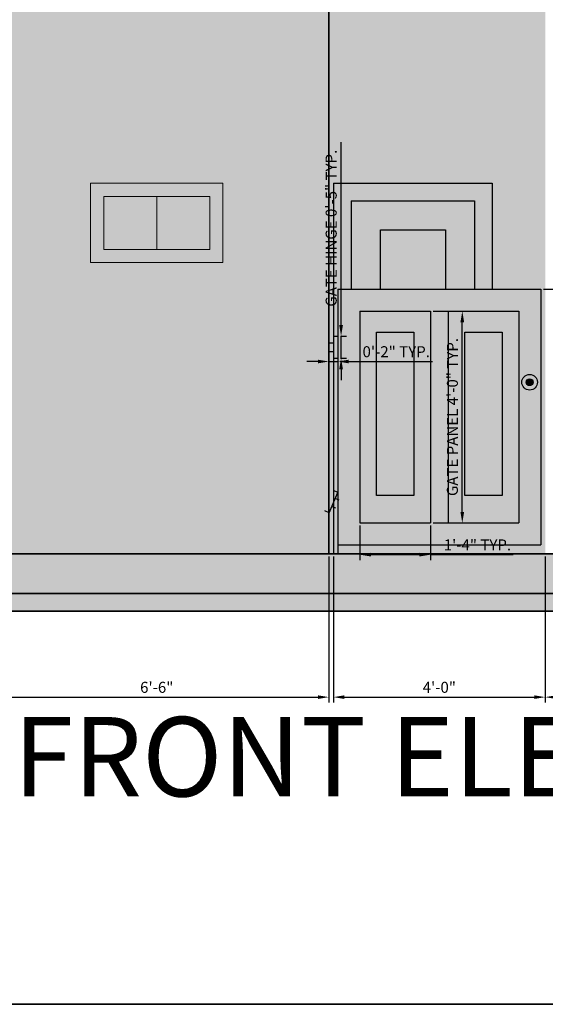
# Model space of a CAD drawing. Units: inches. Extents: x 2150 to 10686, y 1035 to 5077.
# Tile 6 of 12: x 6249 to 6368, y 4201 to 4425. Entities that reach past the tile are written whole.
import ezdxf

# ---------------------------------------------------------------- set-up
doc = ezdxf.new("R2010")
doc.units = ezdxf.units.IN
for name, color, linetype, lineweight in [('A-ANNO-DIMS', 2, 'Continuous', 18), ('A-ANNO-TITL', 3, 'Continuous', 35), ('A-ANNO-TTLB', 7, 'Continuous', 35), ('A-ELEV', 7, 'Continuous', 35), ('A-ELEV-BASE-PATT', 251, 'Continuous', 13), ('A-ELEV-DOOR', 7, 'Continuous', 25), ('A-ELEV-DOOR-PATT', 17, 'Continuous', 13), ('A-ELEV-GLAZ', 7, 'Continuous', 18), ('A-ELEV-METL-PATT', 252, 'Continuous', 13)]:
    doc.layers.add(name, color=color, linetype=linetype, lineweight=lineweight)
doc.layers.add('A-ELEV-GLAZ-PATT', color=141, linetype='Continuous', lineweight=13, true_color=0xadddf7)
doc.layers.add('A-ELEV-PATT', color=253, linetype='Continuous', lineweight=13, true_color=0xa5adc8)
doc.styles.get("Standard").update_dxf_attribs({"font": 'arial.ttf'})
doc.dimstyles.new('ISO-25', dxfattribs={"dimtxt": 2.5, "dimasz": 2.5, "dimexe": 1.25, "dimexo": 0.625, "dimtad": 1, "dimdec": 0, "dimlunit": 3, "dimtxsty": 'Standard', "dimcen": 2.5, "dimadec": 0, "dimazin": 0, "dimtfac": 1, "dimtdec": 0, "dimtmove": 0, "dimatfit": 3, "dimfxl": 1, "dimarcsym": 0})

# ---------------------------------------------------------------- blocks, each defined once
blk = doc.blocks.new('GATE-INSET-PANEL-16')
for p, q in [((-0.0003365621996636, 48.00046013132396), (15.99966343780033, 48.00046013132396)), ((-0.0003365621987541, 48.00046013132396), (-0.0003365622005731, 0.0004601313230523)), ((15.99966343780033, 48.00046013132396), (15.99966343780033, 0.0004601313239618)), ((-0.0003365622005731, 0.0004601313239618), (15.99966343780033, 0.0004601313239618))]:
    blk.add_line(p, q)
blk.add_lwpolyline([(3.788000571435077, 43.25048342382524), (12.21132630416559, 43.25048342382524), (12.21132630416559, 6.206833629573338), (3.788000571435077, 6.206833629573338)], close=True)
blk = doc.blocks.new('GATE-HINGE-5IN')
for p, q in [((0.9996634378003363, 5.000328444739352), (1.999663437801245, 5.000328444739352)), ((0.9996634378003363, 5.000328444739352), (0.9996634378003363, 0.0003284447393526)), ((-0.0003365622005731, 3.500328444739352), (0.9996634378003363, 3.500328444739352)), ((-0.0003365622005731, 1.500328444739352), (0.9996634378003363, 1.500328444739352)), ((0.9996634378003363, 0.0003284447402621), (1.999663437801245, 0.0003284447393526))]:
    blk.add_line(p, q)
blk = doc.blocks.new('*D72')
at = {"layer": 'A-ANNO-DIMS', "color": 0, "lineweight": -2, "transparency": 16777216}
for p, q in [((6342.232663437805, 4358.484460131326), (6350.057663437808, 4358.484460131326)), ((6348.807663437807, 4312.984460131325), (6348.807663437807, 4355.984460131327)), ((6342.232663437805, 4310.484460131325), (6350.057663437808, 4310.484460131325))]:
    blk.add_line(p, q, dxfattribs=at)
at = {"layer": 'A-ANNO-DIMS', "color": 0, "transparency": 16777216}
for points in [[(6348.39099677114, 4355.984460131327), (6349.224330104474, 4355.984460131327), (6348.807663437807, 4358.484460131326)], [(6348.39099677114, 4312.984460131325), (6349.224330104474, 4312.984460131325), (6348.807663437807, 4310.484460131325)]]:
    blk.add_solid(points, dxfattribs=at)
at = {"layer": 'Defpoints', "color": 0, "transparency": 16777216}
for p in [(6341.607663437804, 4358.484460131326), (6348.807663437807, 4358.484460131326), (6341.607663437804, 4310.484460131325)]:
    blk.add_point(p, dxfattribs=at)
at = {"layer": 'A-ANNO-DIMS', "color": 0, "transparency": 16777216, "insert": (6346.8900304228, 4334.484460131323), "char_height": 2.5, "attachment_point": 5, "rotation": 90}
blk.add_mtext('GATE PANEL 4\'-0" TYP.', dxfattribs=at)
blk = doc.blocks.new('*D73')
at = {"layer": 'A-ANNO-DIMS', "color": 0, "lineweight": -2, "transparency": 16777216}
for p, q in [((6325.6076634378, 4309.859460131323), (6325.6076634378, 4302.034460131323)), ((6341.607663437801, 4309.859460131323), (6341.607663437801, 4302.034460131323)), ((6328.107663437799, 4303.284460131323), (6339.1076634378, 4303.284460131323)), ((6341.607663437801, 4303.284460131323), (6360.361074079001, 4303.284460131323))]:
    blk.add_line(p, q, dxfattribs=at)
at = {"layer": 'A-ANNO-DIMS', "color": 0, "transparency": 16777216}
for points in [[(6328.107663437799, 4303.70112679799), (6328.107663437799, 4302.867793464656), (6325.6076634378, 4303.284460131323)], [(6339.1076634378, 4303.70112679799), (6339.1076634378, 4302.867793464656), (6341.607663437801, 4303.284460131323)]]:
    blk.add_solid(points, dxfattribs=at)
at = {"layer": 'Defpoints', "color": 0, "transparency": 16777216}
for p in [(6325.6076634378, 4310.484460131323), (6341.607663437801, 4310.484460131323), (6341.607663437801, 4303.284460131323)]:
    blk.add_point(p, dxfattribs=at)
at = {"layer": 'A-ANNO-DIMS', "color": 0, "transparency": 16777216, "insert": (6352.2343687584, 4305.165428753425), "char_height": 2.5, "attachment_point": 5}
blk.add_mtext('1\'-4" TYP.', dxfattribs=at)
blk = doc.blocks.new('*D76')
at = {"layer": 'A-ANNO-DIMS', "color": 0, "lineweight": -2, "transparency": 16777216}
for p, q in [((6321.35766343781, 4355.313328444741), (6321.35766343781, 4396.771377557974)), ((6321.232663437806, 4352.813328444741), (6322.60766343781, 4352.813328444741)), ((6321.35766343781, 4347.813328444741), (6321.35766343781, 4352.813328444741)), ((6321.232663437806, 4347.813328444741), (6322.60766343781, 4347.813328444741)), ((6321.35766343781, 4345.313328444741), (6321.35766343781, 4342.813328444741))]:
    blk.add_line(p, q, dxfattribs=at)
at = {"layer": 'A-ANNO-DIMS', "color": 0, "transparency": 16777216}
for points in [[(6320.940996771143, 4355.313328444741), (6321.774330104477, 4355.313328444741), (6321.35766343781, 4352.813328444741)], [(6320.940996771143, 4345.313328444741), (6321.774330104477, 4345.313328444741), (6321.35766343781, 4347.813328444741)]]:
    blk.add_solid(points, dxfattribs=at)
at = {"layer": 'Defpoints', "color": 0, "transparency": 16777216}
for p in [(6320.607663437806, 4352.813328444741), (6321.35766343781, 4352.813328444741), (6320.607663437806, 4347.813328444741)]:
    blk.add_point(p, dxfattribs=at)
at = {"layer": 'A-ANNO-DIMS', "color": 0, "transparency": 16777216, "insert": (6319.440030422802, 4377.292353001354), "char_height": 2.5, "attachment_point": 5, "rotation": 90}
blk.add_mtext('GATE HINGE 0\'-5" TYP.', dxfattribs=at)
blk = doc.blocks.new('*D77')
at = {"layer": 'A-ANNO-DIMS', "color": 0, "lineweight": -2, "transparency": 16777216}
for p, q in [((6316.107663437801, 4347.063328444739), (6313.6076634378, 4347.063328444739)), ((6318.6076634378, 4347.188328444739), (6318.6076634378, 4345.813328444739)), ((6318.6076634378, 4347.063328444739), (6320.607663437802, 4347.063328444739)), ((6320.607663437802, 4347.188328444739), (6320.607663437802, 4345.813328444739)), ((6323.107663437802, 4347.063328444739), (6342.09640832184, 4347.063328444739))]:
    blk.add_line(p, q, dxfattribs=at)
at = {"layer": 'A-ANNO-DIMS', "color": 0, "transparency": 16777216}
for points in [[(6316.107663437801, 4347.479995111406), (6316.107663437801, 4346.646661778073), (6318.6076634378, 4347.063328444739)], [(6323.107663437802, 4347.479995111406), (6323.107663437802, 4346.646661778073), (6320.607663437802, 4347.063328444739)]]:
    blk.add_solid(points, dxfattribs=at)
at = {"layer": 'Defpoints', "color": 0, "transparency": 16777216}
for p in [(6318.6076634378, 4347.813328444739), (6320.607663437802, 4347.813328444739), (6320.607663437802, 4347.063328444739)]:
    blk.add_point(p, dxfattribs=at)
at = {"layer": 'A-ANNO-DIMS', "color": 0, "transparency": 16777216, "insert": (6333.852035879822, 4348.964760914044), "char_height": 2.5, "attachment_point": 5}
blk.add_mtext('0\'-2" TYP.', dxfattribs=at)
blk = doc.blocks.new('*D127')
at = {"layer": 'A-ANNO-DIMS', "color": 0, "lineweight": -2, "transparency": 16777216}
for p, q in [((6336.982663000004, 4554.484460000002), (6207.857663000007, 4554.484460000002)), ((6209.107663000008, 4292.984460000002), (6209.107663000008, 4551.984460000001)), ((6233.982663000003, 4290.484460000001), (6207.857663000007, 4290.484460000001))]:
    blk.add_line(p, q, dxfattribs=at)
at = {"layer": 'A-ANNO-DIMS', "color": 0, "transparency": 16777216}
for points in [[(6208.69099633334, 4551.984460000001), (6209.524329666674, 4551.984460000001), (6209.107663000008, 4554.484460000002)], [(6208.69099633334, 4292.984460000002), (6209.524329666674, 4292.984460000002), (6209.107663000008, 4290.484460000001)]]:
    blk.add_solid(points, dxfattribs=at)
at = {"layer": 'Defpoints', "color": 0, "transparency": 16777216}
for p in [(6209.107663000008, 4554.484460000002), (6337.607663000003, 4554.484460000002), (6234.607663000003, 4290.484460000001)]:
    blk.add_point(p, dxfattribs=at)
at = {"layer": 'A-ANNO-DIMS', "color": 0, "transparency": 16777216, "insert": (6207.206230530702, 4422.484459999998), "char_height": 2.5, "attachment_point": 5, "rotation": 90}
blk.add_mtext('22\'-0"', dxfattribs=at)
blk = doc.blocks.new('*D134')
at = {"layer": 'A-ANNO-DIMS', "color": 0, "lineweight": -2, "transparency": 16777216}
for p, q in [((6240.607663, 4302.859459999999), (6240.607663, 4269.73446)), ((6318.607663, 4302.859459999999), (6318.607663, 4269.73446)), ((6243.107662999999, 4270.98446), (6316.107663, 4270.98446))]:
    blk.add_line(p, q, dxfattribs=at)
at = {"layer": 'A-ANNO-DIMS', "color": 0, "transparency": 16777216}
for points in [[(6243.107662999999, 4271.401126666666), (6243.107662999999, 4270.567793333333), (6240.607663, 4270.98446)], [(6316.107663, 4271.401126666666), (6316.107663, 4270.567793333333), (6318.607663, 4270.98446)]]:
    blk.add_solid(points, dxfattribs=at)
at = {"layer": 'Defpoints', "color": 0, "transparency": 16777216}
for p in [(6240.607663, 4303.484459999999), (6318.607663, 4303.484459999999), (6318.607663, 4270.98446)]:
    blk.add_point(p, dxfattribs=at)
at = {"layer": 'A-ANNO-DIMS', "color": 0, "transparency": 16777216, "insert": (6279.607663, 4272.885892469304), "char_height": 2.5, "attachment_point": 5}
blk.add_mtext('6\'-6"', dxfattribs=at)
blk = doc.blocks.new('*D135')
at = {"layer": 'A-ANNO-DIMS', "color": 0, "lineweight": -2, "transparency": 16777216}
for p, q in [((6367.607663, 4302.859459999999), (6367.607663, 4269.73446)), ((6480.607662999999, 4302.859459999999), (6480.607662999999, 4269.73446)), ((6370.107662999999, 4270.98446), (6478.107663, 4270.98446))]:
    blk.add_line(p, q, dxfattribs=at)
at = {"layer": 'A-ANNO-DIMS', "color": 0, "transparency": 16777216}
for points in [[(6370.107662999999, 4271.401126666666), (6370.107662999999, 4270.567793333333), (6367.607663, 4270.98446)], [(6478.107663, 4271.401126666666), (6478.107663, 4270.567793333333), (6480.607662999999, 4270.98446)]]:
    blk.add_solid(points, dxfattribs=at)
at = {"layer": 'Defpoints', "color": 0, "transparency": 16777216}
for p in [(6367.607663, 4303.484459999999), (6480.607662999999, 4303.484459999999), (6480.607662999999, 4270.98446)]:
    blk.add_point(p, dxfattribs=at)
at = {"layer": 'A-ANNO-DIMS', "color": 0, "transparency": 16777216, "insert": (6424.107663, 4272.885892469304), "char_height": 2.5, "attachment_point": 5}
blk.add_mtext('9\'-5"', dxfattribs=at)
blk = doc.blocks.new('*D136')
at = {"layer": 'A-ANNO-DIMS', "color": 0, "lineweight": -2, "transparency": 16777216}
for p, q in [((6319.607663, 4302.859459999999), (6319.607663, 4269.73446)), ((6367.607663, 4302.859459999999), (6367.607663, 4269.73446)), ((6322.107663, 4270.98446), (6365.107662999999, 4270.98446))]:
    blk.add_line(p, q, dxfattribs=at)
at = {"layer": 'A-ANNO-DIMS', "color": 0, "transparency": 16777216}
for points in [[(6322.107663, 4271.401126666666), (6322.107663, 4270.567793333333), (6319.607663, 4270.98446)], [(6365.107662999999, 4271.401126666666), (6365.107662999999, 4270.567793333333), (6367.607663, 4270.98446)]]:
    blk.add_solid(points, dxfattribs=at)
at = {"layer": 'Defpoints', "color": 0, "transparency": 16777216}
for p in [(6319.607663, 4303.484459999999), (6367.607663, 4303.484459999999), (6367.607663, 4270.98446)]:
    blk.add_point(p, dxfattribs=at)
at = {"layer": 'A-ANNO-DIMS', "color": 0, "transparency": 16777216, "insert": (6343.607663, 4272.885892469304), "char_height": 2.5, "attachment_point": 5}
blk.add_mtext('4\'-0"', dxfattribs=at)
blk = doc.blocks.new('*D137')
at = {"layer": 'A-ANNO-DIMS', "color": 0, "lineweight": -2, "transparency": 16777216}
for p, q in [((6367.232663000003, 4363.484460000001), (6513.357663000007, 4363.484460000001)), ((6512.107663000008, 4305.984460000001), (6512.107663000008, 4360.984460000001)), ((6368.232663000004, 4303.484460000001), (6513.357663000007, 4303.484460000001))]:
    blk.add_line(p, q, dxfattribs=at)
at = {"layer": 'A-ANNO-DIMS', "color": 0, "transparency": 16777216}
for points in [[(6511.69099633334, 4360.984460000001), (6512.524329666674, 4360.984460000001), (6512.107663000008, 4363.484460000001)], [(6511.69099633334, 4305.984460000001), (6512.524329666674, 4305.984460000001), (6512.107663000008, 4303.484460000001)]]:
    blk.add_solid(points, dxfattribs=at)
at = {"layer": 'Defpoints', "color": 0, "transparency": 16777216}
for p in [(6366.607663000003, 4363.484460000001), (6512.107663000008, 4363.484460000001), (6367.607663000003, 4303.484460000001)]:
    blk.add_point(p, dxfattribs=at)
at = {"layer": 'A-ANNO-DIMS', "color": 0, "transparency": 16777216, "insert": (6510.206230530702, 4333.484459999999), "char_height": 2.5, "attachment_point": 5, "rotation": 90}
blk.add_mtext('5\'-0"', dxfattribs=at)

msp = doc.modelspace()

# ---------------------------------------------------------------- hatches: boundary and pattern name
at = {"layer": 'A-ELEV-BASE-PATT'}
h = msp.add_hatch(color=256, dxfattribs=at)
h.dxf.hatch_style = 1
h.paths.add_polyline_path([(6480.633239304355, 4303.484460131323), (6240.6076634378, 4303.484460131323), (6240.6076634378, 4294.484460131323), (6480.633239304355, 4294.484460131323)])
h = msp.add_hatch(color=256, dxfattribs=at)
h.dxf.hatch_style = 1
h.paths.add_polyline_path([(6486.607663437801, 4294.484460131323), (6234.607663437801, 4294.484460131323), (6234.607663437801, 4290.484460131323), (6486.6076634378, 4290.484460131323)])
at = {"layer": 'A-ELEV-DOOR-PATT'}
h = msp.add_hatch(color=256, dxfattribs=at)
h.dxf.hatch_style = 1
h.paths.add_polyline_path([(6355.607663437799, 4387.484460131323), (6319.607663437802, 4387.484460131323), (6319.607663437796, 4352.813328444739), (6320.607663437801, 4352.813328444739), (6320.607663437801, 4363.484460131323), (6323.607663437798, 4363.484460131323), (6323.607663437799, 4383.484460131323), (6351.607663437799, 4383.484460131323), (6351.6076634378, 4363.484460131324), (6355.607663437799, 4363.484460131324)])
h.paths.add_polyline_path([(6345.020548115272, 4376.933312986706), (6330.255677554148, 4376.933312986706), (6330.255677554148, 4363.484460131323), (6345.020548115272, 4363.484460131324)], flags=17)
h = msp.add_hatch(color=256, dxfattribs=at)
h.dxf.hatch_style = 1
h.paths.add_polyline_path([(6351.607663437799, 4383.484460131323), (6323.607663437799, 4383.484460131323), (6323.607663437798, 4363.484460131323), (6330.255677554148, 4363.484460131323), (6330.255677554148, 4376.933312986706), (6345.020548115272, 4376.933312986706), (6345.020548115272, 4363.484460131324), (6351.6076634378, 4363.484460131324)])
h = msp.add_hatch(color=256, dxfattribs=at)
h.dxf.hatch_style = 1
h.paths.add_polyline_path([(6366.607663437799, 4363.484460131324), (6320.607663437801, 4363.484460131323), (6320.6076634378, 4305.484460131324), (6366.6076634378, 4305.484460131324)])
h.paths.add_polyline_path([(6341.607663437801, 4358.484460131324), (6341.607663437801, 4310.484460131324), (6325.6076634378, 4310.484460131324), (6325.607663437802, 4358.484460131324)], flags=16)
h.paths.add_polyline_path([(6329.396000571435, 4353.734483423825), (6337.819326304166, 4353.734483423825), (6337.819326304166, 4316.690833629574), (6329.396000571435, 4316.690833629574)], flags=0)
h.paths.add_polyline_path([(6345.6076634378, 4358.484460131324), (6361.6076634378, 4358.484460131324), (6361.6076634378, 4310.484460131323), (6345.6076634378, 4310.484460131324)], flags=16)
h.paths.add_polyline_path([(6349.396000571435, 4353.734483423825), (6357.819326304166, 4353.734483423825), (6357.819326304166, 4316.690833629574), (6349.396000571435, 4316.690833629574)], flags=0)
h.paths.add_polyline_path([(6365.841192765556, 4342.374498147924, -1), (6362.290894053427, 4342.374498147924, -1)], flags=16)
h.paths.add_polyline_path([(6364.841192765556, 4342.374498147924, -1), (6363.290894053427, 4342.374498147924, -1)], flags=0)
h.paths.add_polyline_path([(6337.819326304166, 4353.734483423825), (6329.396000571435, 4353.734483423825), (6329.396000571435, 4316.690833629574), (6337.819326304166, 4316.690833629574)], flags=0)
h = msp.add_hatch(color=256, dxfattribs=at)
h.dxf.hatch_style = 1
h.paths.add_polyline_path([(6320.607663437801, 4347.813328444739), (6319.607663437796, 4347.81332844474), (6319.607663437793, 4317.600749510185), (6320.6076634378, 4317.600749510185)])
h.paths.add_polyline_path([(6320.6076634378, 4312.600749510185), (6319.607663437793, 4312.600749510185), (6319.607663437792, 4303.484460131323), (6320.6076634378, 4303.484460131323)])
at = {"layer": 'A-ELEV-GLAZ-PATT'}
h = msp.add_hatch(color=256, dxfattribs=at)
h.dxf.hatch_style = 1
h.paths.add_polyline_path([(6279.607663437801, 4384.484460131323), (6267.607663437801, 4384.484460131323), (6267.6076634378, 4372.484460131324), (6279.607663437801, 4372.484460131324)])
h.paths.add_polyline_path([(6291.607663437801, 4384.484460131323), (6279.607663437801, 4384.484460131323), (6279.607663437801, 4372.484460131324), (6291.607663437801, 4372.484460131324)])
edge = h.paths.add_edge_path()
edge.add_ellipse((6400.444858416264, 4425.167712730096), major_axis=(0, -62.64324057997146), ratio=0.3301887017017349, start_angle=180.9156291084783, end_angle=267.2317619230999)
edge.add_line((6379.76340377621, 4426.167712730096), (6399.444858416265, 4426.167712730096))
edge.add_line((6399.444858416265, 4426.167712730096), (6399.444858416265, 4487.737700317675))
edge = h.paths.add_edge_path()
edge.add_ellipse((6400.444858416264, 4425.167712730096), major_axis=(0, -62.64324057997146), ratio=0.3301887017017349, start_angle=452.7682380769, end_angle=539.0843708915216)
edge.add_line((6401.444858416265, 4487.737700317675), (6401.444858416265, 4426.167712730096))
edge.add_line((6401.444858416265, 4426.167712730096), (6421.126313056319, 4426.167712730096))
edge = h.paths.add_edge_path()
edge.add_ellipse((6400.444858416264, 4425.167712730096), major_axis=(0, -62.64324057997146), ratio=0.3301887017017349, start_angle=378.88994340641, end_angle=447.2317619231)
edge.add_line((6421.126313056319, 4424.167712730096), (6401.444858416265, 4424.167712730096))
edge.add_line((6401.444858416265, 4424.167712730096), (6401.444858416265, 4376.02078865707))
edge.add_line((6401.444858416265, 4376.02078865707), (6408.633239304354, 4376.02078865707))
edge.add_line((6408.633239304354, 4376.02078865707), (6408.633239304354, 4382.020788657071))
edge.add_line((6408.633239304354, 4382.020788657071), (6415.329204846509, 4381.669182122283))
edge = h.paths.add_edge_path()
edge.add_line((6399.444858416265, 4424.167712730096), (6379.76340377621, 4424.167712730096))
edge.add_ellipse((6400.444858416264, 4425.167712730096), major_axis=(0, -62.64324057997146), ratio=0.3301887017017349, start_angle=272.7682380768999, end_angle=349.9116256040723)
edge.add_line((6390.633239304354, 4370.020788657071), (6399.444858416265, 4370.020788657071))
edge.add_line((6399.444858416265, 4370.020788657071), (6399.444858416265, 4424.167712730096))
edge = h.paths.add_edge_path()
edge.add_line((6399.444858416265, 4370.020788657071), (6390.633239304354, 4370.020788657071))
edge.add_ellipse((6400.444858416264, 4425.167712730096), major_axis=(0, -62.64324057997146), ratio=0.3301887017017349, start_angle=349.9116256040723, end_angle=359.0843708915216)
edge.add_line((6399.444858416265, 4362.597725142516), (6399.444858416265, 4370.020788657071))
edge = h.paths.add_edge_path()
edge.add_ellipse((6400.444858416264, 4425.167712730096), major_axis=(0, -62.64324057997146), ratio=0.3301887017017349, start_angle=360.9156291084783, end_angle=378.88994340641)
edge.add_line((6415.329204846509, 4381.669182122283), (6408.633239304354, 4382.020788657071))
edge.add_line((6408.633239304354, 4382.020788657071), (6408.633239304354, 4376.02078865707))
edge.add_line((6408.633239304354, 4376.02078865707), (6401.444858416265, 4376.02078865707))
edge.add_line((6401.444858416265, 4376.02078865707), (6401.444858416265, 4362.597725142516))
at = {"layer": 'A-ELEV-METL-PATT'}
h = msp.add_hatch(color=256, dxfattribs=at)
h.dxf.hatch_style = 1
edge = h.paths.add_edge_path()
edge.add_spline(control_points=[(6400.444858416264, 4358.524472150125), (6401.486440814489, 4358.524472150125), (6402.526505044808, 4358.677401357236), (6404.522486905328, 4359.255063234454), (6405.478003331038, 4359.677509034017), (6407.281736042183, 4360.731176144923), (6408.131339490663, 4361.361806443027), (6409.740207013673, 4362.793659380537), (6410.500149994661, 4363.595296803934), (6412.700838569434, 4366.265752912591), (6414.03394570237, 4368.379499630626), (6416.487744706213, 4373.197243253772), (6417.606172835956, 4375.903063890813), (6419.631029857393, 4381.840607040826), (6420.536486327513, 4385.072192199597), (6422.117938633519, 4391.962202533656), (6422.793588111736, 4395.620342382234), (6424.200323950252, 4405.332886237875), (6424.756775730746, 4411.600724829638), (6425.233072301224, 4424.345165291339), (6425.152698848673, 4430.819672112305), (6424.360861114452, 4443.427756971612), (6423.649784349251, 4449.559211921115), (6421.832101343849, 4459.914160022554), (6420.824100186611, 4464.280479948769), (6418.459699862937, 4472.224057176997), (6417.105531965493, 4475.800577784561), (6414.530984821721, 4481.046021704659), (6413.400413444257, 4482.963765924061), (6411.159609652, 4486.022314366695), (6410.081239671351, 4487.242292157316), (6407.981904490796, 4489.103336574784), (6406.994481886034, 4489.812440503778), (6404.88004816331, 4490.945334575583), (6403.750412373089, 4491.367263683768), (6401.591707320996, 4491.795744529485), (6400.578062848126, 4491.856564882596), (6398.574329452856, 4491.695615966483), (6397.586567833659, 4491.47475953499), (6395.700279883302, 4490.794741309719), (6394.801423289315, 4490.337316033343), (6393.101630982474, 4489.237707960262), (6392.299575991901, 4488.59571921333), (6390.776032761522, 4487.156246990203), (6390.054097434259, 4486.358390989495), (6387.868726596746, 4483.603993381065), (6386.519519142056, 4481.381571183187), (6384.042618140686, 4476.318979222956), (6382.917389359787, 4473.477169667343), (6380.892123096994, 4467.249882245213), (6379.993066323842, 4463.864616669574), (6378.439918554827, 4456.661812920038), (6377.786169577303, 4452.844597947903), (6376.462930365054, 4442.788115239438), (6375.974391004774, 4436.347147441612), (6375.659764204387, 4423.32378833974), (6375.833828926627, 4416.743682061819), (6376.8313878542, 4404.020783955098), (6377.654325200822, 4397.880344812312), (6379.642069279475, 4387.821914067098), (6380.689035460468, 4383.713325470128), (6383.106877716371, 4376.272307259607), (6384.47532253611, 4372.940336073535), (6387.048331366607, 4368.105027158752), (6388.164220640812, 4366.356485480582), (6390.369702204264, 4363.581332383819), (6391.427944586487, 4362.479757644216), (6393.496381316636, 4360.802633777571), (6394.475915167926, 4360.166036636088), (6396.563807655099, 4359.173441496676), (6397.674090126379, 4358.819701830231), (6399.355629057865, 4358.565786838256), (6399.900211293723, 4358.524472150125), (6400.444858416264, 4358.524472150125)], knot_values=[0, 0, 0, 0, 0.0952714022776172, 0.0952714022776172, 0.1905428045552344, 0.1905428045552344, 0.2858142068328516, 0.2858142068328516, 0.3810856091104688, 0.3810856091104688, 0.575169634462188, 0.575169634462188, 0.7692536598139071, 0.7692536598139071, 0.9633376851656262, 0.9633376851656262, 1.157421710517345, 1.157421710517345, 1.458089536658081, 1.458089536658081, 1.758757362798818, 1.758757362798818, 2.059425188939554, 2.059425188939554, 2.304413142887573, 2.304413142887573, 2.549401096835591, 2.549401096835591, 2.718168677128249, 2.718168677128249, 2.856837524264077, 2.856837524264077, 2.966492349551455, 2.966492349551455, 3.076147174838833, 3.076147174838833, 3.168108685177037, 3.168108685177037, 3.260070195515242, 3.260070195515242, 3.352031705853447, 3.352031705853447, 3.443993216191651, 3.443993216191651, 3.535954726529856, 3.535954726529856, 3.735259798893268, 3.735259798893268, 3.93456487125668, 3.93456487125668, 4.133869943620092, 4.133869943620092, 4.333175015983504, 4.333175015983504, 4.639352924429541, 4.639352924429541, 4.945530832875578, 4.945530832875578, 5.251708741321616, 5.251708741321616, 5.489766878495931, 5.489766878495931, 5.727825015670246, 5.727825015670246, 5.88940932659502, 5.88940932659502, 6.02159730311115, 6.02159730311115, 6.127482428421133, 6.127482428421133, 6.233367553731117, 6.233367553731117, 6.283185307179586, 6.283185307179586, 6.283185307179586, 6.283185307179586], degree=3, periodic=0)
edge = h.paths.add_edge_path(flags=16)
edge.add_line((6399.444858416265, 4487.737700317675), (6399.444858416265, 4426.167712730096))
edge.add_line((6399.444858416265, 4426.167712730096), (6379.76340377621, 4426.167712730096))
edge.add_ellipse((6400.444858416264, 4425.167712730096), major_axis=(0, -62.64324057997146), ratio=0.3301887017017349, start_angle=180.9156291084783, end_angle=267.2317619230999, ccw=False)
edge = h.paths.add_edge_path(flags=16)
edge.add_ellipse((6400.444858416264, 4425.167712730096), major_axis=(0, -62.64324057997146), ratio=0.3301887017017349, start_angle=452.7682380769001, end_angle=539.0843708915218, ccw=False)
edge.add_line((6421.126313056319, 4426.167712730096), (6401.444858416265, 4426.167712730096))
edge.add_line((6401.444858416265, 4426.167712730096), (6401.444858416265, 4487.737700317675))
edge = h.paths.add_edge_path(flags=16)
edge.add_line((6399.444858416265, 4424.167712730097), (6399.444858416265, 4370.020788657071))
edge.add_line((6399.444858416265, 4370.020788657071), (6399.633239304353, 4370.020788657071))
edge.add_line((6399.633239304353, 4370.020788657071), (6399.633239304353, 4376.02078865707))
edge.add_line((6399.633239304353, 4376.02078865707), (6401.444858416265, 4376.02078865707))
edge.add_line((6401.444858416265, 4376.02078865707), (6401.444858416265, 4424.167712730096))
edge.add_line((6401.444858416265, 4424.167712730096), (6421.126313056319, 4424.167712730096))
edge.add_ellipse((6400.444858416264, 4425.167712730096), major_axis=(0, -62.64324057997146), ratio=0.3301887017017349, start_angle=378.88994340641005, end_angle=447.23176192310007, ccw=False)
edge.add_ellipse((6400.444858416264, 4425.167712730096), major_axis=(0, -62.64324057997146), ratio=0.3301887017017349, start_angle=360.9156291084783, end_angle=378.88994340641005, ccw=False)
edge.add_line((6401.444858416265, 4362.597725142516), (6401.444858416265, 4376.02078865707))
edge.add_line((6401.444858416265, 4376.02078865707), (6399.633239304353, 4376.02078865707))
edge.add_line((6399.633239304353, 4376.02078865707), (6399.633239304353, 4370.020788657071))
edge.add_line((6399.633239304353, 4370.020788657071), (6399.444858416265, 4370.020788657071))
edge.add_line((6399.444858416265, 4370.020788657071), (6399.444858416265, 4362.597725142516))
edge.add_ellipse((6400.444858416264, 4425.167712730096), major_axis=(0, -62.64324057997146), ratio=0.3301887017017349, start_angle=349.9116256040723, end_angle=359.0843708915217, ccw=False)
edge.add_ellipse((6400.444858416264, 4425.167712730096), major_axis=(0, -62.64324057997146), ratio=0.3301887017017349, start_angle=272.76823807689993, end_angle=349.9116256040723, ccw=False)
edge.add_line((6379.76340377621, 4424.167712730096), (6399.444858416265, 4424.167712730097))
h.paths.add_polyline_path([(6294.607663437801, 4387.484460131323), (6264.6076634378, 4387.484460131323), (6264.6076634378, 4369.484460131324), (6294.607663437801, 4369.484460131324)])
h.paths.add_polyline_path([(6267.607663437801, 4384.484460131323), (6291.607663437801, 4384.484460131323), (6291.607663437801, 4372.484460131324), (6267.6076634378, 4372.484460131324)], flags=16)
h = msp.add_hatch(color=256, dxfattribs=at)
h.dxf.hatch_style = 1
h.paths.add_polyline_path([(6361.6076634378, 4358.484460131324), (6345.6076634378, 4358.484460131324), (6345.6076634378, 4310.484460131324), (6361.6076634378, 4310.484460131323)])
h.paths.add_polyline_path([(6349.396000571435, 4353.734483423825), (6357.819326304166, 4353.734483423825), (6357.819326304166, 4316.690833629574), (6349.396000571435, 4316.690833629574)], flags=16)
h.paths.add_polyline_path([(6341.607663437801, 4358.484460131324), (6325.607663437802, 4358.484460131324), (6325.6076634378, 4310.484460131324), (6341.607663437801, 4310.484460131324)])
h.paths.add_polyline_path([(6337.819326304166, 4353.734483423825), (6337.819326304166, 4316.690833629574), (6329.396000571435, 4316.690833629574), (6329.396000571435, 4353.734483423825)], flags=16)
h.paths.add_polyline_path([(6362.290894053427, 4342.374498147924, 1), (6365.841192765556, 4342.374498147924, 1)])
h.paths.add_polyline_path([(6364.841192765556, 4342.374498147924, -1), (6363.290894053427, 4342.374498147924, -1)], flags=16)
h = msp.add_hatch(color=256, dxfattribs=at)
h.dxf.hatch_style = 1
h.paths.add_polyline_path([(6320.607663437801, 4352.813328444739), (6319.607663437801, 4352.813328444739), (6319.607663437801, 4347.81332844474), (6320.607663437801, 4347.813328444739)])
h.paths.add_polyline_path([(6319.607663437801, 4351.31332844474), (6318.607663437799, 4351.31332844474), (6318.607663437799, 4349.313328444739), (6319.607663437801, 4349.313328444739)])
h.paths.add_polyline_path([(6320.6076634378, 4317.600749510185), (6319.6076634378, 4317.600749510185), (6319.6076634378, 4312.600749510185), (6320.6076634378, 4312.600749510185)])
h.paths.add_polyline_path([(6319.6076634378, 4316.100749510185), (6318.607663437799, 4316.100749510185), (6318.607663437799, 4314.100749510185), (6319.6076634378, 4314.100749510185)])
h.paths.add_polyline_path([(6337.819326304166, 4353.734483423825), (6329.396000571435, 4353.734483423825), (6329.396000571435, 4316.690833629574), (6337.819326304166, 4316.690833629574)])
h.paths.add_polyline_path([(6357.819326304166, 4353.734483423825), (6349.396000571435, 4353.734483423825), (6349.396000571435, 4316.690833629574), (6357.819326304166, 4316.690833629574)])
h = msp.add_hatch(color=256, dxfattribs=at)
h.dxf.hatch_style = 1
h.paths.add_polyline_path([(6364.841192765556, 4342.374498147924, 1), (6363.290894053427, 4342.374498147924, 1)])
at = {"layer": 'A-ELEV-PATT'}
h = msp.add_hatch(color=256, dxfattribs=at)
h.dxf.hatch_style = 1
h.paths.add_polyline_path([(6318.6076634378, 4447.484460131323), (6240.6076634378, 4447.484460131323), (6240.6076634378, 4303.484460131323), (6318.607663437799, 4303.484460131323)])
h.paths.add_polyline_path([(6294.607663437801, 4387.484460131323), (6294.607663437801, 4369.484460131324), (6264.6076634378, 4369.484460131324), (6264.6076634378, 4387.484460131323)], flags=16)
h.paths.add_polyline_path([(6291.607663437801, 4384.484460131324), (6291.607663437801, 4372.484460131324), (6267.6076634378, 4372.484460131324), (6267.607663437801, 4384.484460131323)], flags=0)
h = msp.add_hatch(color=256, dxfattribs=at)
h.dxf.hatch_style = 1
h.paths.add_polyline_path([(6367.6076634378, 4447.484460131323), (6318.6076634378, 4447.484460131323), (6318.607663437799, 4303.484460131323), (6319.607663437792, 4303.484460131323), (6319.607663437802, 4387.484460131323), (6355.607663437799, 4387.484460131323), (6355.607663437799, 4363.484460131324), (6366.607663437799, 4363.484460131324), (6366.6076634378, 4305.484460131324), (6320.6076634378, 4305.484460131324), (6320.6076634378, 4303.484460131323), (6367.6076634378, 4303.484460131323)])

# ---------------------------------------------------------------- linework, layer by layer
at = {"layer": 'A-ANNO-TTLB'}
msp.add_lwpolyline([(6112.690859240117, 5076.611187983804), (7001.249989206184, 5076.611187983804), (7001.249989206184, 4201.352691599126), (6112.690859240117, 4201.352691599126)], close=True, dxfattribs=at)
at = {"layer": 'A-ELEV'}
for p, q in [((6318.6076634378, 4447.484460131323), (6318.607663437799, 4303.484460131323)), ((6240.6076634378, 4303.484460131323), (6480.6076634378, 4303.484460131323)), ((6234.607663437801, 4294.484460131323), (6486.6076634378, 4294.484460131323)), ((6234.607663437801, 4290.484460131323), (6486.6076634378, 4290.484460131323))]:
    msp.add_line(p, q, dxfattribs=at)
at = {"layer": 'A-ELEV-DOOR'}
for p, q in [((6319.607663437802, 4387.484460131323), (6355.607663437799, 4387.484460131323)), ((6319.607663437802, 4387.484460131323), (6319.607663437792, 4303.484460131323)), ((6355.607663437799, 4387.484460131323), (6355.607663437799, 4363.484460131324)), ((6323.607663437798, 4383.484460131323), (6351.6076634378, 4383.484460131323)), ((6323.607663437799, 4383.484460131323), (6323.607663437798, 4363.484460131323)), ((6351.607663437799, 4383.484460131323), (6351.6076634378, 4363.484460131323)), ((6320.607663437801, 4363.484460131323), (6366.607663437799, 4363.484460131324)), ((6320.607663437801, 4363.484460131323), (6320.6076634378, 4303.484460131323)), ((6366.607663437799, 4363.484460131323), (6366.6076634378, 4305.484460131324)), ((6320.607663437801, 4305.484460131324), (6366.6076634378, 4305.484460131324))]:
    msp.add_line(p, q, dxfattribs=at)
msp.add_lwpolyline([(6330.255677554148, 4363.484460131323), (6330.255677554148, 4376.933312986706), (6345.020548115272, 4376.933312986706), (6345.020548115272, 4363.484460131324)], dxfattribs=at)
for radius in [1.775149356064503, 0.7751493560645031]:
    msp.add_circle((6364.066043409492, 4342.374498147924), radius, dxfattribs=at)
at = {"layer": 'A-ELEV-GLAZ'}
for p, q in [((6264.6076634378, 4387.484460131323), (6264.6076634378, 4369.484460131324)), ((6294.607663437801, 4387.484460131323), (6264.6076634378, 4387.484460131323)), ((6294.607663437801, 4387.484460131323), (6294.607663437801, 4369.484460131324)), ((6267.607663437801, 4384.484460131322), (6267.6076634378, 4372.484460131324)), ((6291.607663437801, 4384.484460131323), (6267.607663437801, 4384.484460131323)), ((6279.607663437801, 4384.484460131323), (6279.607663437801, 4372.484460131324)), ((6291.607663437801, 4384.484460131324), (6291.607663437801, 4372.484460131324)), ((6291.607663437801, 4372.484460131324), (6267.6076634378, 4372.484460131324)), ((6294.607663437801, 4369.484460131324), (6264.6076634378, 4369.484460131324))]:
    msp.add_line(p, q, dxfattribs=at)

# ---------------------------------------------------------------- block references
at = {"layer": 'A-ELEV-DOOR'}
for name, p in [('GATE-INSET-PANEL-16', (6325.608, 4310.484)), ('GATE-INSET-PANEL-16', (6345.607999999998, 4310.483999999999)), ('GATE-HINGE-5IN', (6318.608000000001, 4347.813))]:
    msp.add_blockref(name, p, dxfattribs=at)
at = {"layer": 'A-ELEV-DOOR', "rotation": 156.8014094863339}
msp.add_blockref('GATE-HINGE-5IN', (6321.511426745516, 4317.005127253346), dxfattribs=at)

# ---------------------------------------------------------------- texts
at = {"layer": 'A-ANNO-TITL', "insert": (6247.142359601145, 4266.476998592536), "char_height": 18, "attachment_point": 1}
msp.add_mtext_dynamic_manual_height_columns('FRONT ELEVATION', width=338.5750231852289, gutter_width=12.5, heights=[0], dxfattribs=at)

# ---------------------------------------------------------------- dimensions: what is measured, and where the dimension line sits
at = {"layer": 'A-ANNO-DIMS'}
for base, p1, p2, picture, middle in [((6209.107663000008, 4554.484460000002), (6234.607663, 4290.48446), (6337.607663, 4554.48446), '*D127', (6207.206230530702, 4422.484459999998)), ((6512.107663000008, 4363.484460000001), (6367.607663, 4303.484459999999), (6366.607662999999, 4363.48446), '*D137', (6510.206230530702, 4333.484459999999))]:
    dim = msp.add_linear_dim(base=base, p1=p1, p2=p2, angle=90, dimstyle='ISO-25', override={"dimdec": 1, "dimlfac": 1, "dimrnd": 0, "dimzin": 1, "dimdsep": 46, "dimlunit": 4, "dimfrac": 2}, dxfattribs=at)
    dim.commit()
    dim.dimension.update_dxf_attribs({"geometry": picture, "text_midpoint": middle})
for base, p1, p2, text, picture, middle in [((6321.35766343781, 4352.813328444741), (6320.607663437802, 4347.813328444739), (6320.607663437802, 4352.813328444739), 'GATE HINGE <> TYP.', '*D76', (6319.440030422802, 4377.292353001354)), ((6348.807663437807, 4358.484460131326), (6341.607663437801, 4310.484460131323), (6341.607663437801, 4358.484460131324), 'GATE PANEL <> TYP.', '*D72', (6346.8900304228, 4334.484460131323))]:
    dim = msp.add_linear_dim(base=base, p1=p1, p2=p2, angle=90, text=text, dimstyle='ISO-25', override={"dimdec": 1, "dimlfac": 1, "dimrnd": 0, "dimzin": 1, "dimdsep": 46, "dimlunit": 4, "dimfrac": 2}, dxfattribs=at)
    dim.commit()
    dim.dimension.update_dxf_attribs({"geometry": picture, "text_midpoint": middle})
for base, p1, p2, picture, middle in [((6320.607663437802, 4347.063328444739), (6318.6076634378, 4347.813328444739), (6320.607663437802, 4347.813328444739), '*D77', (6333.852035879822, 4348.964760914044)), ((6341.607663437801, 4303.284460131323), (6325.6076634378, 4310.484460131323), (6341.607663437801, 4310.484460131323), '*D73', (6352.2343687584, 4305.165428753425))]:
    dim = msp.add_linear_dim(base=base, p1=p1, p2=p2, text='<> TYP.', dimstyle='ISO-25', override={"dimdec": 1, "dimlfac": 1, "dimrnd": 0, "dimzin": 1, "dimdsep": 46, "dimlunit": 4, "dimfrac": 2}, dxfattribs=at)
    dim.commit()
    dim.dimension.update_dxf_attribs({"geometry": picture, "text_midpoint": middle})
for base, p1, p2, picture, middle in [((6318.607663, 4270.98446), (6240.607663, 4303.484459999999), (6318.607663, 4303.484459999999), '*D134', (6279.607663, 4272.885892469304)), ((6367.607663, 4270.98446), (6319.607663, 4303.484459999999), (6367.607663, 4303.484459999999), '*D136', (6343.607663, 4272.885892469304)), ((6480.607662999999, 4270.98446), (6367.607663, 4303.484459999999), (6480.607662999999, 4303.484459999999), '*D135', (6424.107663, 4272.885892469304))]:
    dim = msp.add_linear_dim(base=base, p1=p1, p2=p2, dimstyle='ISO-25', override={"dimdec": 1, "dimlfac": 1, "dimrnd": 0, "dimzin": 1, "dimdsep": 46, "dimlunit": 4, "dimfrac": 2}, dxfattribs=at)
    dim.commit()
    dim.dimension.update_dxf_attribs({"geometry": picture, "text_midpoint": middle})

doc.saveas('drawing.dxf')
